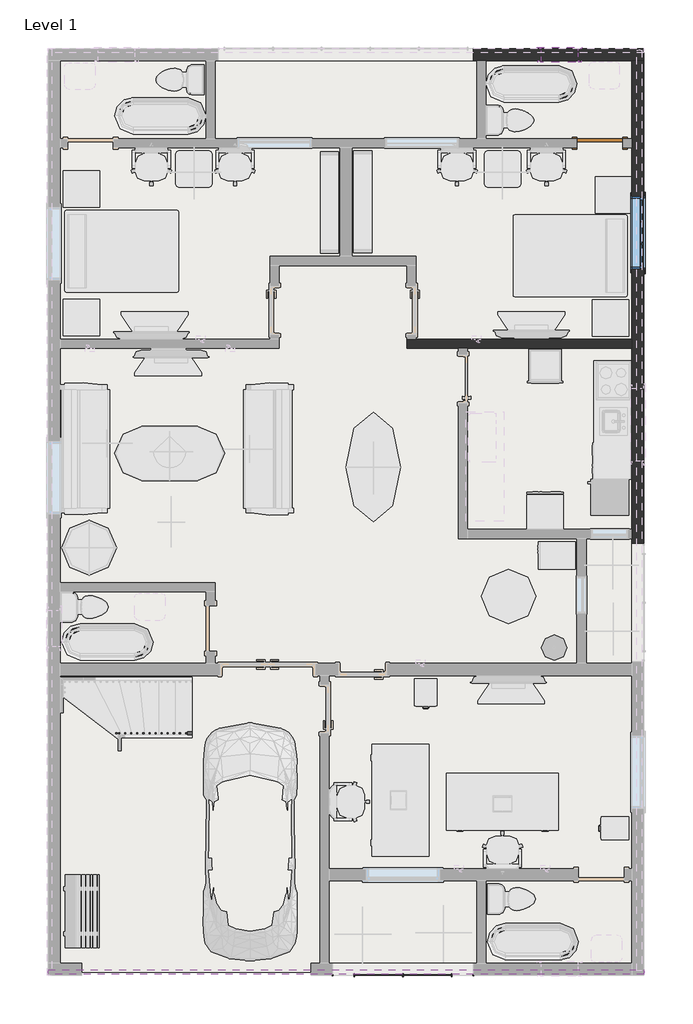
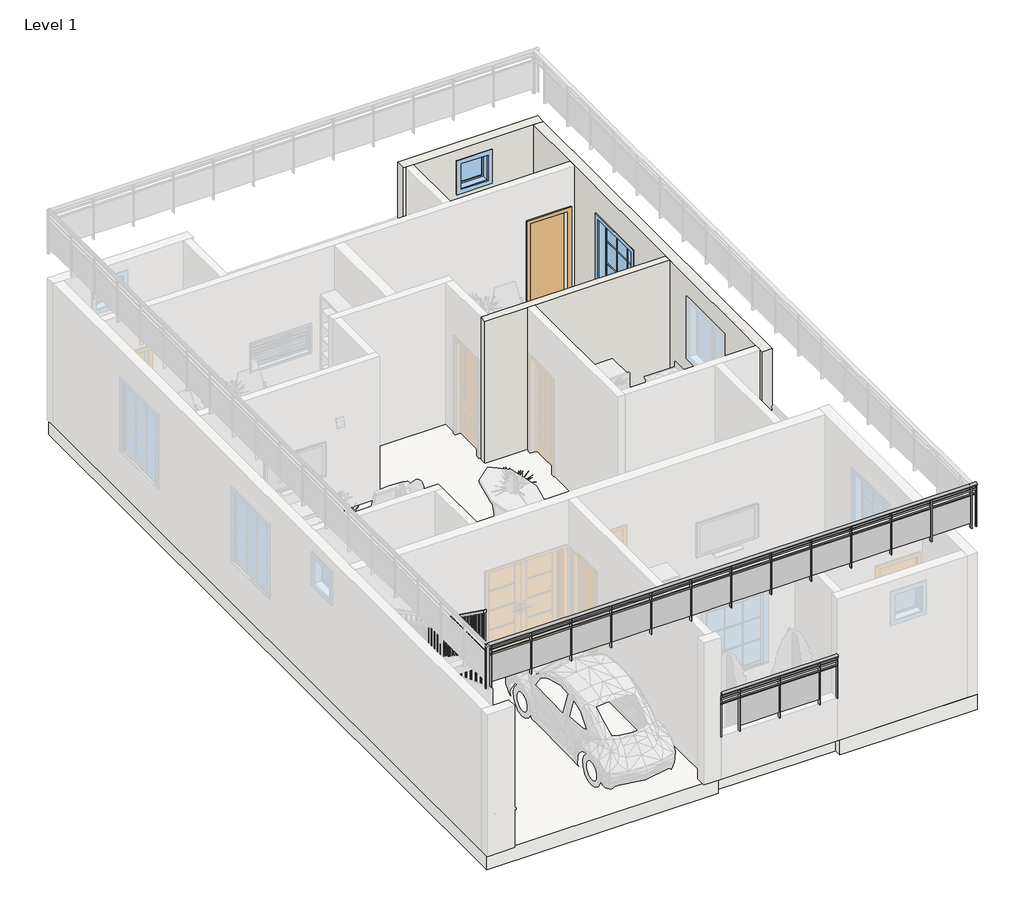
# One storey, part 2 of 5: 3 railings, 3 walls, 2 windows, 1 door, 1 slab.
"""IFC4 building model written with IfcOpenShell, lengths in millimetres."""

from ifc_helpers import new_model, si_unit, point, frame, origin, place, context, project, spatial, polyline, ellipse_curve, trimmed, outline, extrude, faceted_brep, transform, mapped, element, save
from ifc_brep_helpers import plane_surface, extruded_surface, advanced_brep
from components import door_a9addea7, window_cfa1ffdd, window_e41d21a6

model = new_model("IFC4")

# Units and contexts
model_context = context("Model", 3, world=origin())
ifc_project = project(units=[si_unit("LENGTHUNIT", "METRE", prefix="MILLI")], contexts=[model_context])

# Site, building, storey
site = spatial("IfcSite", under=ifc_project)
building = spatial("IfcBuilding", under=site)
storey = spatial("IfcBuildingStorey", under=building, Name="Level 1", Elevation=0.0)

# Door
placement = place(None, origin())
door_shape = door_a9addea7(model_context)
element("IfcDoor", 1, ObjectType="Single-Flush : 30\" x 84\"", at=placement, inside=storey, context=model_context, shape_type="MappedRepresentation", body=[
    mapped(door_shape, transform((1921.0042848, 14492.9691167, 0.0), x_axis=(1.0, 0.0, 0.0), y_axis=(0.0, 1.0, 0.0), z_axis=(0.0, 0.0, 1.0))),
])

# Railings
element("IfcRailing", 2, ObjectType="Glass Panel - Bottom Fill", at=placement, inside=storey, context=model_context, shape_type="SolidModel", body=[
    advanced_brep(
    [(-2549.3957152, 637.2691167, 1828.8), (-2549.3957152, 561.0691167, 1828.8), (-187.1957152, 637.2691167, 1828.8), (-187.1957152, 561.0691167, 1828.8)],
    [
        (0, 1, ellipse_curve(frame((-2549.3957152, 599.1691167, 1828.8), z_axis=(-1.0, 0.0, 0.0), x_axis=(0.0, -1.0, 0.0)), 38.1, 28.575)),
        (1, 0, ellipse_curve(frame((-2549.3957152, 599.1691167, 1828.8), z_axis=(-1.0, 0.0, 0.0), x_axis=(0.0, -1.0, 0.0)), 38.1, 28.575)),
        (2, 3, ellipse_curve(frame((-187.1957152, 599.1691167, 1828.8), z_axis=(1.0, 0.0, 0.0), x_axis=(0.0, -1.0, 0.0)), 38.1, 28.575)),
        (3, 2, ellipse_curve(frame((-187.1957152, 599.1691167, 1828.8), z_axis=(1.0, 0.0, 0.0), x_axis=(0.0, -1.0, 0.0)), 38.1, 28.575)),
        (0, 2),
        (3, 1),
    ],
    [
        plane_surface(frame((-2549.3957152, 599.1691167, 1828.8), z_axis=(-1.0, 0.0, 0.0), x_axis=(0.0, 1.0, 0.0))),
        plane_surface(frame((-187.1957152, 599.1691167, 1828.8), z_axis=(1.0, 0.0, 0.0), x_axis=(0.0, 1.0, 0.0))),
        extruded_surface(trimmed(ellipse_curve(frame((-187.1957152, 599.1691167, 1828.8), z_axis=(-1.0, 0.0, 0.0), x_axis=(0.0, -1.0, 0.0)), 38.1, 28.575), [point((-187.1957152, 637.2691167, 1828.8))], [point((-187.1957152, 561.0691167, 1828.8))], True, "CARTESIAN"), (-2362.2, 0.0, 0.0), 2362.2),
        extruded_surface(trimmed(ellipse_curve(frame((-187.1957152, 599.1691167, 1828.8), z_axis=(-1.0, 0.0, 0.0), x_axis=(0.0, -1.0, 0.0)), 38.1, 28.575), [point((-187.1957152, 561.0691167, 1828.8))], [point((-187.1957152, 637.2691167, 1828.8))], True, "CARTESIAN"), (-2362.2, 0.0, 0.0), 2362.2),
    ],
    [
        (0, [[1, 2]]),
        (1, [[3, 4]]),
        (2, [[-1, 5, -4, 6]]),
        (3, [[-2, -6, -3, -5]]),
    ],
),
    extrude(outline(polyline([(-2549.3957152, 586.4691167), (-2549.3957152, 611.8691167), (-187.1957152, 611.8691167), (-187.1957152, 586.4691167), (-2549.3957152, 586.4691167)])), frame((0.0, 0.0, 1714.5), z_axis=(0.0, 0.0, 1.0), x_axis=(1.0, 0.0, 0.0)), (0.0, 0.0, 1.0), 25.4),
    extrude(outline(polyline([(-2549.3957152, 586.4691167), (-2549.3957152, 611.8691167), (-187.1957152, 611.8691167), (-187.1957152, 586.4691167), (-2549.3957152, 586.4691167)])), frame((0.0, 0.0, 1612.9), z_axis=(0.0, 0.0, 1.0), x_axis=(1.0, 0.0, 0.0)), (0.0, 0.0, 1.0), 25.4),
    extrude(outline(polyline([(-561.8457152, 573.7691167), (-561.8457152, 624.5691167), (-549.1457152, 624.5691167), (-549.1457152, 573.7691167), (-561.8457152, 573.7691167)])), frame((0.0, 0.0, 914.4), z_axis=(0.0, 0.0, 1.0), x_axis=(1.0, 0.0, 0.0)), (0.0, 0.0, 1.0), 885.6788223),
    extrude(outline(polyline([(-1368.2957152, 605.7042737), (-555.4957152, 605.7042737), (-555.4957152, 599.3542737), (-1368.2957152, 599.3542737), (-1368.2957152, 605.7042737)])), frame((0.0, 0.0, 1016.0), z_axis=(0.0, 0.0, 1.0), x_axis=(1.0, 0.0, 0.0)), (0.0, 0.0, 1.0), 596.9),
    extrude(outline(polyline([(-1374.6457152, 573.7691167), (-1374.6457152, 624.5691167), (-1361.9457152, 624.5691167), (-1361.9457152, 573.7691167), (-1374.6457152, 573.7691167)])), frame((0.0, 0.0, 914.4), z_axis=(0.0, 0.0, 1.0), x_axis=(1.0, 0.0, 0.0)), (0.0, 0.0, 1.0), 885.6788223),
    extrude(outline(polyline([(-2181.0957152, 605.7042737), (-1368.2957152, 605.7042737), (-1368.2957152, 599.3542737), (-2181.0957152, 599.3542737), (-2181.0957152, 605.7042737)])), frame((0.0, 0.0, 1016.0), z_axis=(0.0, 0.0, 1.0), x_axis=(1.0, 0.0, 0.0)), (0.0, 0.0, 1.0), 596.9),
    extrude(outline(polyline([(-2187.4457152, 573.7691167), (-2187.4457152, 624.5691167), (-2174.7457152, 624.5691167), (-2174.7457152, 573.7691167), (-2187.4457152, 573.7691167)])), frame((0.0, 0.0, 914.4), z_axis=(0.0, 0.0, 1.0), x_axis=(1.0, 0.0, 0.0)), (0.0, 0.0, 1.0), 885.6788223),
    extrude(outline(polyline([(-199.8957152, 589.6441167), (-199.8957152, 608.6941167), (-180.8457152, 608.6941167), (-180.8457152, 589.6441167), (-199.8957152, 589.6441167)])), frame((0.0, 0.0, 914.4), z_axis=(0.0, 0.0, 1.0), x_axis=(1.0, 0.0, 0.0)), (0.0, 0.0, 1.0), 885.6788223),
    extrude(outline(polyline([(-2555.7457152, 589.6441167), (-2555.7457152, 608.6941167), (-2536.6957152, 608.6941167), (-2536.6957152, 589.6441167), (-2555.7457152, 589.6441167)])), frame((0.0, 0.0, 914.4), z_axis=(0.0, 0.0, 1.0), x_axis=(1.0, 0.0, 0.0)), (0.0, 0.0, 1.0), 885.6788223),
])
element("IfcRailing", 3, ObjectType="Glass Panel - Bottom Fill", at=placement, inside=storey, context=model_context, shape_type="SolidModel", body=[
    advanced_brep(
    [(-7299.1957152, 688.0691167, 4495.8), (-7299.1957152, 611.8691167, 4495.8), (2657.6042848, 688.0691167, 4495.8), (2657.6042848, 611.8691167, 4495.8)],
    [
        (0, 1, ellipse_curve(frame((-7299.1957152, 649.9691167, 4495.8), z_axis=(-1.0, 0.0, 0.0), x_axis=(0.0, -1.0, 0.0)), 38.1, 28.575)),
        (1, 0, ellipse_curve(frame((-7299.1957152, 649.9691167, 4495.8), z_axis=(-1.0, 0.0, 0.0), x_axis=(0.0, -1.0, 0.0)), 38.1, 28.575)),
        (2, 3, ellipse_curve(frame((2657.6042848, 649.9691167, 4495.8), z_axis=(1.0, 0.0, 0.0), x_axis=(0.0, -1.0, 0.0)), 38.1, 28.575)),
        (3, 2, ellipse_curve(frame((2657.6042848, 649.9691167, 4495.8), z_axis=(1.0, 0.0, 0.0), x_axis=(0.0, -1.0, 0.0)), 38.1, 28.575)),
        (0, 2),
        (3, 1),
    ],
    [
        plane_surface(frame((-7299.1957152, 649.9691167, 4495.8), z_axis=(-1.0, 0.0, 0.0), x_axis=(0.0, 1.0, 0.0))),
        plane_surface(frame((2657.6042848, 649.9691167, 4495.8), z_axis=(1.0, 0.0, 0.0), x_axis=(0.0, 1.0, 0.0))),
        extruded_surface(trimmed(ellipse_curve(frame((2657.6042848, 649.9691167, 4495.8), z_axis=(-1.0, 0.0, 0.0), x_axis=(0.0, -1.0, 0.0)), 38.1, 28.575), [point((2657.6042848, 688.0691167, 4495.8))], [point((2657.6042848, 611.8691167, 4495.8))], True, "CARTESIAN"), (-9956.800000000001, 0.0, 0.0), 9956.800000000001),
        extruded_surface(trimmed(ellipse_curve(frame((2657.6042848, 649.9691167, 4495.8), z_axis=(-1.0, 0.0, 0.0), x_axis=(0.0, -1.0, 0.0)), 38.1, 28.575), [point((2657.6042848, 611.8691167, 4495.8))], [point((2657.6042848, 688.0691167, 4495.8))], True, "CARTESIAN"), (-9956.800000000001, 0.0, 0.0), 9956.800000000001),
    ],
    [
        (0, [[1, 2]]),
        (1, [[3, 4]]),
        (2, [[-1, 5, -4, 6]]),
        (3, [[-2, -6, -3, -5]]),
    ],
),
    extrude(outline(polyline([(-7299.1957152, 637.2691167), (-7299.1957152, 662.6691167), (2657.6042848, 662.6691167), (2657.6042848, 637.2691167), (-7299.1957152, 637.2691167)])), frame((0.0, 0.0, 4381.5), z_axis=(0.0, 0.0, 1.0), x_axis=(1.0, 0.0, 0.0)), (0.0, 0.0, 1.0), 25.4),
    extrude(outline(polyline([(-7299.1957152, 637.2691167), (-7299.1957152, 662.6691167), (2657.6042848, 662.6691167), (2657.6042848, 637.2691167), (-7299.1957152, 637.2691167)])), frame((0.0, 0.0, 4279.9), z_axis=(0.0, 0.0, 1.0), x_axis=(1.0, 0.0, 0.0)), (0.0, 0.0, 1.0), 25.4),
    extrude(outline(polyline([(2549.6542848, 624.5691167), (2549.6542848, 675.3691167), (2562.3542848, 675.3691167), (2562.3542848, 624.5691167), (2549.6542848, 624.5691167)])), frame((0.0, 0.0, 3581.4), z_axis=(0.0, 0.0, 1.0), x_axis=(1.0, 0.0, 0.0)), (0.0, 0.0, 1.0), 885.6788223),
    extrude(outline(polyline([(1743.2042848, 656.5042737), (2556.0042848, 656.5042737), (2556.0042848, 650.1542737), (1743.2042848, 650.1542737), (1743.2042848, 656.5042737)])), frame((0.0, 0.0, 3683.0), z_axis=(0.0, 0.0, 1.0), x_axis=(1.0, 0.0, 0.0)), (0.0, 0.0, 1.0), 596.9),
    extrude(outline(polyline([(1736.8542848, 624.5691167), (1736.8542848, 675.3691167), (1749.5542848, 675.3691167), (1749.5542848, 624.5691167), (1736.8542848, 624.5691167)])), frame((0.0, 0.0, 3581.4), z_axis=(0.0, 0.0, 1.0), x_axis=(1.0, 0.0, 0.0)), (0.0, 0.0, 1.0), 885.6788223),
    extrude(outline(polyline([(930.4042848, 656.5042737), (1743.2042848, 656.5042737), (1743.2042848, 650.1542737), (930.4042848, 650.1542737), (930.4042848, 656.5042737)])), frame((0.0, 0.0, 3683.0), z_axis=(0.0, 0.0, 1.0), x_axis=(1.0, 0.0, 0.0)), (0.0, 0.0, 1.0), 596.9),
    extrude(outline(polyline([(924.0542848, 624.5691167), (924.0542848, 675.3691167), (936.7542848, 675.3691167), (936.7542848, 624.5691167), (924.0542848, 624.5691167)])), frame((0.0, 0.0, 3581.4), z_axis=(0.0, 0.0, 1.0), x_axis=(1.0, 0.0, 0.0)), (0.0, 0.0, 1.0), 885.6788223),
    extrude(outline(polyline([(117.6042848, 656.5042737), (930.4042848, 656.5042737), (930.4042848, 650.1542737), (117.6042848, 650.1542737), (117.6042848, 656.5042737)])), frame((0.0, 0.0, 3683.0), z_axis=(0.0, 0.0, 1.0), x_axis=(1.0, 0.0, 0.0)), (0.0, 0.0, 1.0), 596.9),
    extrude(outline(polyline([(111.2542848, 624.5691167), (111.2542848, 675.3691167), (123.9542848, 675.3691167), (123.9542848, 624.5691167), (111.2542848, 624.5691167)])), frame((0.0, 0.0, 3581.4), z_axis=(0.0, 0.0, 1.0), x_axis=(1.0, 0.0, 0.0)), (0.0, 0.0, 1.0), 885.6788223),
    extrude(outline(polyline([(-695.1957152, 656.5042737), (117.6042848, 656.5042737), (117.6042848, 650.1542737), (-695.1957152, 650.1542737), (-695.1957152, 656.5042737)])), frame((0.0, 0.0, 3683.0), z_axis=(0.0, 0.0, 1.0), x_axis=(1.0, 0.0, 0.0)), (0.0, 0.0, 1.0), 596.9),
    extrude(outline(polyline([(-701.5457152, 624.5691167), (-701.5457152, 675.3691167), (-688.8457152, 675.3691167), (-688.8457152, 624.5691167), (-701.5457152, 624.5691167)])), frame((0.0, 0.0, 3581.4), z_axis=(0.0, 0.0, 1.0), x_axis=(1.0, 0.0, 0.0)), (0.0, 0.0, 1.0), 885.6788223),
    extrude(outline(polyline([(-1507.9957152, 656.5042737), (-695.1957152, 656.5042737), (-695.1957152, 650.1542737), (-1507.9957152, 650.1542737), (-1507.9957152, 656.5042737)])), frame((0.0, 0.0, 3683.0), z_axis=(0.0, 0.0, 1.0), x_axis=(1.0, 0.0, 0.0)), (0.0, 0.0, 1.0), 596.9),
    extrude(outline(polyline([(-1514.3457152, 624.5691167), (-1514.3457152, 675.3691167), (-1501.6457152, 675.3691167), (-1501.6457152, 624.5691167), (-1514.3457152, 624.5691167)])), frame((0.0, 0.0, 3581.4), z_axis=(0.0, 0.0, 1.0), x_axis=(1.0, 0.0, 0.0)), (0.0, 0.0, 1.0), 885.6788223),
    extrude(outline(polyline([(-2320.7957152, 656.5042737), (-1507.9957152, 656.5042737), (-1507.9957152, 650.1542737), (-2320.7957152, 650.1542737), (-2320.7957152, 656.5042737)])), frame((0.0, 0.0, 3683.0), z_axis=(0.0, 0.0, 1.0), x_axis=(1.0, 0.0, 0.0)), (0.0, 0.0, 1.0), 596.9),
    extrude(outline(polyline([(-2327.1457152, 624.5691167), (-2327.1457152, 675.3691167), (-2314.4457152, 675.3691167), (-2314.4457152, 624.5691167), (-2327.1457152, 624.5691167)])), frame((0.0, 0.0, 3581.4), z_axis=(0.0, 0.0, 1.0), x_axis=(1.0, 0.0, 0.0)), (0.0, 0.0, 1.0), 885.6788223),
    extrude(outline(polyline([(-3133.5957152, 656.5042737), (-2320.7957152, 656.5042737), (-2320.7957152, 650.1542737), (-3133.5957152, 650.1542737), (-3133.5957152, 656.5042737)])), frame((0.0, 0.0, 3683.0), z_axis=(0.0, 0.0, 1.0), x_axis=(1.0, 0.0, 0.0)), (0.0, 0.0, 1.0), 596.9),
    extrude(outline(polyline([(-3139.9457152, 624.5691167), (-3139.9457152, 675.3691167), (-3127.2457152, 675.3691167), (-3127.2457152, 624.5691167), (-3139.9457152, 624.5691167)])), frame((0.0, 0.0, 3581.4), z_axis=(0.0, 0.0, 1.0), x_axis=(1.0, 0.0, 0.0)), (0.0, 0.0, 1.0), 885.6788223),
    extrude(outline(polyline([(-3946.3957152, 656.5042737), (-3133.5957152, 656.5042737), (-3133.5957152, 650.1542737), (-3946.3957152, 650.1542737), (-3946.3957152, 656.5042737)])), frame((0.0, 0.0, 3683.0), z_axis=(0.0, 0.0, 1.0), x_axis=(1.0, 0.0, 0.0)), (0.0, 0.0, 1.0), 596.9),
    extrude(outline(polyline([(-3952.7457152, 624.5691167), (-3952.7457152, 675.3691167), (-3940.0457152, 675.3691167), (-3940.0457152, 624.5691167), (-3952.7457152, 624.5691167)])), frame((0.0, 0.0, 3581.4), z_axis=(0.0, 0.0, 1.0), x_axis=(1.0, 0.0, 0.0)), (0.0, 0.0, 1.0), 885.6788223),
    extrude(outline(polyline([(-4759.1957152, 656.5042737), (-3946.3957152, 656.5042737), (-3946.3957152, 650.1542737), (-4759.1957152, 650.1542737), (-4759.1957152, 656.5042737)])), frame((0.0, 0.0, 3683.0), z_axis=(0.0, 0.0, 1.0), x_axis=(1.0, 0.0, 0.0)), (0.0, 0.0, 1.0), 596.9),
    extrude(outline(polyline([(-4765.5457152, 624.5691167), (-4765.5457152, 675.3691167), (-4752.8457152, 675.3691167), (-4752.8457152, 624.5691167), (-4765.5457152, 624.5691167)])), frame((0.0, 0.0, 3581.4), z_axis=(0.0, 0.0, 1.0), x_axis=(1.0, 0.0, 0.0)), (0.0, 0.0, 1.0), 885.6788223),
    extrude(outline(polyline([(-5571.9957152, 656.5042737), (-4759.1957152, 656.5042737), (-4759.1957152, 650.1542737), (-5571.9957152, 650.1542737), (-5571.9957152, 656.5042737)])), frame((0.0, 0.0, 3683.0), z_axis=(0.0, 0.0, 1.0), x_axis=(1.0, 0.0, 0.0)), (0.0, 0.0, 1.0), 596.9),
    extrude(outline(polyline([(-5578.3457152, 624.5691167), (-5578.3457152, 675.3691167), (-5565.6457152, 675.3691167), (-5565.6457152, 624.5691167), (-5578.3457152, 624.5691167)])), frame((0.0, 0.0, 3581.4), z_axis=(0.0, 0.0, 1.0), x_axis=(1.0, 0.0, 0.0)), (0.0, 0.0, 1.0), 885.6788223),
    extrude(outline(polyline([(-6384.7957152, 656.5042737), (-5571.9957152, 656.5042737), (-5571.9957152, 650.1542737), (-6384.7957152, 650.1542737), (-6384.7957152, 656.5042737)])), frame((0.0, 0.0, 3683.0), z_axis=(0.0, 0.0, 1.0), x_axis=(1.0, 0.0, 0.0)), (0.0, 0.0, 1.0), 596.9),
    extrude(outline(polyline([(-6391.1457152, 624.5691167), (-6391.1457152, 675.3691167), (-6378.4457152, 675.3691167), (-6378.4457152, 624.5691167), (-6391.1457152, 624.5691167)])), frame((0.0, 0.0, 3581.4), z_axis=(0.0, 0.0, 1.0), x_axis=(1.0, 0.0, 0.0)), (0.0, 0.0, 1.0), 885.6788223),
    extrude(outline(polyline([(-7197.5957152, 656.5042737), (-6384.7957152, 656.5042737), (-6384.7957152, 650.1542737), (-7197.5957152, 650.1542737), (-7197.5957152, 656.5042737)])), frame((0.0, 0.0, 3683.0), z_axis=(0.0, 0.0, 1.0), x_axis=(1.0, 0.0, 0.0)), (0.0, 0.0, 1.0), 596.9),
    extrude(outline(polyline([(-7203.9457152, 624.5691167), (-7203.9457152, 675.3691167), (-7191.2457152, 675.3691167), (-7191.2457152, 624.5691167), (-7203.9457152, 624.5691167)])), frame((0.0, 0.0, 3581.4), z_axis=(0.0, 0.0, 1.0), x_axis=(1.0, 0.0, 0.0)), (0.0, 0.0, 1.0), 885.6788223),
    extrude(outline(polyline([(2644.9042848, 640.4441167), (2644.9042848, 659.4941167), (2663.9542848, 659.4941167), (2663.9542848, 640.4441167), (2644.9042848, 640.4441167)])), frame((0.0, 0.0, 3581.4), z_axis=(0.0, 0.0, 1.0), x_axis=(1.0, 0.0, 0.0)), (0.0, 0.0, 1.0), 885.6788223),
    extrude(outline(polyline([(-7305.5457152, 640.4441167), (-7305.5457152, 659.4941167), (-7286.4957152, 659.4941167), (-7286.4957152, 640.4441167), (-7305.5457152, 640.4441167)])), frame((0.0, 0.0, 3581.4), z_axis=(0.0, 0.0, 1.0), x_axis=(1.0, 0.0, 0.0)), (0.0, 0.0, 1.0), 885.6788223),
])
element("IfcRailing", 4, ObjectType="Handrail - Rectangular", at=placement, inside=storey, context=model_context, shape_type="SolidModel", body=[
    faceted_brep([(-4892.6027934, 4612.3691167, 1210.6955174), (-4892.6027934, 4612.3691167, 1146.9597126), (-4892.6027934, 4663.1691167, 1146.9597126), (-4892.6027934, 4663.1691167, 1210.6955174), (-6054.5957152, 4612.3691167, 2091.1504574), (-6105.3957152, 4612.3691167, 2065.9063766), (-6105.3957152, 4663.1691167, 2065.9063766), (-6054.5957152, 4663.1691167, 2091.1504574), (-6054.5957152, 4612.3691167, 2301.2616873), (-6105.3957152, 4612.3691167, 2250.4616873), (-6105.3957152, 4663.1691167, 2250.4616873), (-6054.5957152, 4663.1691167, 2301.2616873), (-6130.7957152, 4612.3691167, 2301.2616873), (-6130.7957152, 4612.3691167, 2250.4616873), (-6181.5957152, 4663.1691167, 2250.4616873), (-6181.5957152, 4663.1691167, 2301.2616873), (-6130.7957152, 4536.1691167, 2301.2616873), (-6130.7957152, 4519.8580772, 2250.4616873), (-6181.5957152, 4519.8580772, 2250.4616873), (-6181.5957152, 4536.1691167, 2301.2616873), (-6130.7957152, 2646.197182, 3654.4449888), (-6181.5957152, 2646.197182, 3654.4449888), (-6181.5957152, 2646.197182, 3591.9666004), (-6130.7957152, 2646.197182, 3591.9666004)], [[[0, 1, 2, 3]], [[1, 0, 4, 5]], [[2, 1, 5, 6]], [[3, 2, 6, 7]], [[0, 3, 7, 4]], [[5, 4, 8, 9]], [[6, 5, 9, 10]], [[7, 6, 10, 11]], [[4, 7, 11, 8]], [[9, 8, 12, 13]], [[10, 9, 13, 14]], [[11, 10, 14, 15]], [[8, 11, 15, 12]], [[13, 12, 16, 17]], [[14, 13, 17, 18]], [[15, 14, 18, 19]], [[12, 15, 19, 16]], [[20, 21, 22, 23]], [[17, 16, 20, 23]], [[18, 17, 23, 22]], [[19, 18, 22, 21]], [[16, 19, 21, 20]]]),
    extrude(outline(polyline([(2716.8941167, 3541.3489644), (2716.8941167, 2540.0), (2697.8441167, 2540.0), (2697.8441167, 3554.9883955), (2716.8941167, 3541.3489644)])), frame((-6165.7207152, 0.0, 0.0), z_axis=(1.0, 0.0, 0.0), x_axis=(0.0, 1.0, 0.0)), (0.0, 0.0, 1.0), 19.05),
    extrude(outline(polyline([(2818.4941167, 3468.6053322), (2818.4941167, 2540.0), (2799.4441167, 2540.0), (2799.4441167, 3482.2447632), (2818.4941167, 3468.6053322)])), frame((-6165.7207152, 0.0, 0.0), z_axis=(1.0, 0.0, 0.0), x_axis=(0.0, 1.0, 0.0)), (0.0, 0.0, 1.0), 19.05),
    extrude(outline(polyline([(2920.0941167, 3395.8616999), (2920.0941167, 2540.0), (2901.0441167, 2540.0), (2901.0441167, 3409.5011309), (2920.0941167, 3395.8616999)])), frame((-6165.7207152, 0.0, 0.0), z_axis=(1.0, 0.0, 0.0), x_axis=(0.0, 1.0, 0.0)), (0.0, 0.0, 1.0), 19.05),
    extrude(outline(polyline([(3021.6941167, 3323.1180676), (3021.6941167, 2370.6666667), (3002.6441167, 2370.6666667), (3002.6441167, 3336.7574987), (3021.6941167, 3323.1180676)])), frame((-6165.7207152, 0.0, 0.0), z_axis=(1.0, 0.0, 0.0), x_axis=(0.0, 1.0, 0.0)), (0.0, 0.0, 1.0), 19.05),
    extrude(outline(polyline([(3123.2941167, 3250.3744353), (3123.2941167, 2370.6666667), (3104.2441167, 2370.6666667), (3104.2441167, 3264.0138664), (3123.2941167, 3250.3744353)])), frame((-6165.7207152, 0.0, 0.0), z_axis=(1.0, 0.0, 0.0), x_axis=(0.0, 1.0, 0.0)), (0.0, 0.0, 1.0), 19.05),
    extrude(outline(polyline([(3224.8941167, 3177.6308031), (3224.8941167, 2201.3333333), (3205.8441167, 2201.3333333), (3205.8441167, 3191.2702341), (3224.8941167, 3177.6308031)])), frame((-6165.7207152, 0.0, 0.0), z_axis=(1.0, 0.0, 0.0), x_axis=(0.0, 1.0, 0.0)), (0.0, 0.0, 1.0), 19.05),
    extrude(outline(polyline([(3326.4941167, 3104.8871708), (3326.4941167, 2201.3333333), (3307.4441167, 2201.3333333), (3307.4441167, 3118.5266018), (3326.4941167, 3104.8871708)])), frame((-6165.7207152, 0.0, 0.0), z_axis=(1.0, 0.0, 0.0), x_axis=(0.0, 1.0, 0.0)), (0.0, 0.0, 1.0), 19.05),
    extrude(outline(polyline([(3428.0941167, 3032.1435385), (3428.0941167, 2201.3333333), (3409.0441167, 2201.3333333), (3409.0441167, 3045.7829696), (3428.0941167, 3032.1435385)])), frame((-6165.7207152, 0.0, 0.0), z_axis=(1.0, 0.0, 0.0), x_axis=(0.0, 1.0, 0.0)), (0.0, 0.0, 1.0), 19.05),
    extrude(outline(polyline([(3529.6941167, 2959.3999062), (3529.6941167, 2032.0), (3510.6441167, 2032.0), (3510.6441167, 2973.0393373), (3529.6941167, 2959.3999062)])), frame((-6165.7207152, 0.0, 0.0), z_axis=(1.0, 0.0, 0.0), x_axis=(0.0, 1.0, 0.0)), (0.0, 0.0, 1.0), 19.05),
    extrude(outline(polyline([(3631.2941167, 2886.656274), (3631.2941167, 2032.0), (3612.2441167, 2032.0), (3612.2441167, 2900.295705), (3631.2941167, 2886.656274)])), frame((-6165.7207152, 0.0, 0.0), z_axis=(1.0, 0.0, 0.0), x_axis=(0.0, 1.0, 0.0)), (0.0, 0.0, 1.0), 19.05),
    extrude(outline(polyline([(3732.8941167, 2813.9126417), (3732.8941167, 2032.0), (3713.8441167, 2032.0), (3713.8441167, 2827.5520727), (3732.8941167, 2813.9126417)])), frame((-6165.7207152, 0.0, 0.0), z_axis=(1.0, 0.0, 0.0), x_axis=(0.0, 1.0, 0.0)), (0.0, 0.0, 1.0), 19.05),
    extrude(outline(polyline([(3834.4941167, 2741.1690094), (3834.4941167, 1862.6666667), (3815.4441167, 1862.6666667), (3815.4441167, 2754.8084405), (3834.4941167, 2741.1690094)])), frame((-6165.7207152, 0.0, 0.0), z_axis=(1.0, 0.0, 0.0), x_axis=(0.0, 1.0, 0.0)), (0.0, 0.0, 1.0), 19.05),
    extrude(outline(polyline([(3936.0941167, 2668.4253771), (3936.0941167, 1862.6666667), (3917.0441167, 1862.6666667), (3917.0441167, 2682.0648082), (3936.0941167, 2668.4253771)])), frame((-6165.7207152, 0.0, 0.0), z_axis=(1.0, 0.0, 0.0), x_axis=(0.0, 1.0, 0.0)), (0.0, 0.0, 1.0), 19.05),
    extrude(outline(polyline([(4037.6941167, 2595.6817449), (4037.6941167, 1693.3333333), (4018.6441167, 1693.3333333), (4018.6441167, 2609.3211759), (4037.6941167, 2595.6817449)])), frame((-6165.7207152, 0.0, 0.0), z_axis=(1.0, 0.0, 0.0), x_axis=(0.0, 1.0, 0.0)), (0.0, 0.0, 1.0), 19.05),
    extrude(outline(polyline([(4139.2941167, 2522.9381126), (4139.2941167, 1693.3333333), (4120.2441167, 1693.3333333), (4120.2441167, 2536.5775436), (4139.2941167, 2522.9381126)])), frame((-6165.7207152, 0.0, 0.0), z_axis=(1.0, 0.0, 0.0), x_axis=(0.0, 1.0, 0.0)), (0.0, 0.0, 1.0), 19.05),
    extrude(outline(polyline([(4240.8941167, 2450.1944803), (4240.8941167, 1524.0), (4221.8441167, 1524.0), (4221.8441167, 2463.8339114), (4240.8941167, 2450.1944803)])), frame((-6165.7207152, 0.0, 0.0), z_axis=(1.0, 0.0, 0.0), x_axis=(0.0, 1.0, 0.0)), (0.0, 0.0, 1.0), 19.05),
    extrude(outline(polyline([(4342.4941167, 2377.450848), (4342.4941167, 1524.0), (4323.4441167, 1524.0), (4323.4441167, 2391.0902791), (4342.4941167, 2377.450848)])), frame((-6165.7207152, 0.0, 0.0), z_axis=(1.0, 0.0, 0.0), x_axis=(0.0, 1.0, 0.0)), (0.0, 0.0, 1.0), 19.05),
    extrude(outline(polyline([(4444.0941167, 2304.7072158), (4444.0941167, 1354.6666667), (4425.0441167, 1354.6666667), (4425.0441167, 2318.3466468), (4444.0941167, 2304.7072158)])), frame((-6165.7207152, 0.0, 0.0), z_axis=(1.0, 0.0, 0.0), x_axis=(0.0, 1.0, 0.0)), (0.0, 0.0, 1.0), 19.05),
    extrude(outline(polyline([(-6146.6707152, 4545.6941167), (-6146.6707152, 4526.6441167), (-6165.7207152, 4526.6441167), (-6165.7207152, 4545.6941167), (-6146.6707152, 4545.6941167)])), frame((0.0, 0.0, 1354.6666667), z_axis=(0.0, 0.0, 1.0), x_axis=(1.0, 0.0, 0.0)), (0.0, 0.0, 1.0), 895.7950207),
    extrude(outline(polyline([(2077.8270257, -6121.3277934), (1185.3333333, -6121.3277934), (1185.3333333, -6102.2777934), (2063.3926292, -6102.2777934), (2077.8270257, -6121.3277934)])), frame((0.0, 4628.2441167, 0.0), z_axis=(0.0, 1.0, 0.0), x_axis=(0.0, 0.0, 1.0)), (0.0, 0.0, 1.0), 19.05),
    extrude(outline(polyline([(2000.994841, -6019.7277934), (1016.0, -6019.7277934), (1016.0, -6000.6777934), (1986.5604445, -6000.6777934), (2000.994841, -6019.7277934)])), frame((0.0, 4628.2441167, 0.0), z_axis=(0.0, 1.0, 0.0), x_axis=(0.0, 0.0, 1.0)), (0.0, 0.0, 1.0), 19.05),
    extrude(outline(polyline([(1924.0113928, -5918.1277934), (1016.0, -5918.1277934), (1016.0, -5899.0777934), (1909.5769963, -5899.0777934), (1924.0113928, -5918.1277934)])), frame((0.0, 4628.2441167, 0.0), z_axis=(0.0, 1.0, 0.0), x_axis=(0.0, 0.0, 1.0)), (0.0, 0.0, 1.0), 19.05),
    extrude(outline(polyline([(1847.0279446, -5816.5277934), (846.6666667, -5816.5277934), (846.6666667, -5797.4777934), (1832.5935481, -5797.4777934), (1847.0279446, -5816.5277934)])), frame((0.0, 4628.2441167, 0.0), z_axis=(0.0, 1.0, 0.0), x_axis=(0.0, 0.0, 1.0)), (0.0, 0.0, 1.0), 19.05),
    extrude(outline(polyline([(1770.0444964, -5714.9277934), (846.6666667, -5714.9277934), (846.6666667, -5695.8777934), (1755.6100999, -5695.8777934), (1770.0444964, -5714.9277934)])), frame((0.0, 4628.2441167, 0.0), z_axis=(0.0, 1.0, 0.0), x_axis=(0.0, 0.0, 1.0)), (0.0, 0.0, 1.0), 19.05),
    extrude(outline(polyline([(1693.0610482, -5613.3277934), (677.3333333, -5613.3277934), (677.3333333, -5594.2777934), (1678.6266517, -5594.2777934), (1693.0610482, -5613.3277934)])), frame((0.0, 4628.2441167, 0.0), z_axis=(0.0, 1.0, 0.0), x_axis=(0.0, 0.0, 1.0)), (0.0, 0.0, 1.0), 19.05),
    extrude(outline(polyline([(1616.0776, -5511.7277934), (677.3333333, -5511.7277934), (677.3333333, -5492.6777934), (1601.6432035, -5492.6777934), (1616.0776, -5511.7277934)])), frame((0.0, 4628.2441167, 0.0), z_axis=(0.0, 1.0, 0.0), x_axis=(0.0, 0.0, 1.0)), (0.0, 0.0, 1.0), 19.05),
    extrude(outline(polyline([(1539.0941518, -5410.1277934), (508.0, -5410.1277934), (508.0, -5391.0777934), (1524.6597553, -5391.0777934), (1539.0941518, -5410.1277934)])), frame((0.0, 4628.2441167, 0.0), z_axis=(0.0, 1.0, 0.0), x_axis=(0.0, 0.0, 1.0)), (0.0, 0.0, 1.0), 19.05),
    extrude(outline(polyline([(1462.1107036, -5308.5277934), (508.0, -5308.5277934), (508.0, -5289.4777934), (1447.6763071, -5289.4777934), (1462.1107036, -5308.5277934)])), frame((0.0, 4628.2441167, 0.0), z_axis=(0.0, 1.0, 0.0), x_axis=(0.0, 0.0, 1.0)), (0.0, 0.0, 1.0), 19.05),
    extrude(outline(polyline([(1385.1272554, -5206.9277934), (508.0, -5206.9277934), (508.0, -5187.8777934), (1370.6928589, -5187.8777934), (1385.1272554, -5206.9277934)])), frame((0.0, 4628.2441167, 0.0), z_axis=(0.0, 1.0, 0.0), x_axis=(0.0, 0.0, 1.0)), (0.0, 0.0, 1.0), 19.05),
    extrude(outline(polyline([(1308.1438072, -5105.3277934), (338.6666667, -5105.3277934), (338.6666667, -5086.2777934), (1293.7094107, -5086.2777934), (1308.1438072, -5105.3277934)])), frame((0.0, 4628.2441167, 0.0), z_axis=(0.0, 1.0, 0.0), x_axis=(0.0, 0.0, 1.0)), (0.0, 0.0, 1.0), 19.05),
    extrude(outline(polyline([(1231.160359, -5003.7277934), (338.6666667, -5003.7277934), (338.6666667, -4984.6777934), (1216.7259625, -4984.6777934), (1231.160359, -5003.7277934)])), frame((0.0, 4628.2441167, 0.0), z_axis=(0.0, 1.0, 0.0), x_axis=(0.0, 0.0, 1.0)), (0.0, 0.0, 1.0), 19.05),
    extrude(outline(polyline([(-6146.6707152, 4647.2941167), (-6146.6707152, 4628.2441167), (-6165.7207152, 4628.2441167), (-6165.7207152, 4647.2941167), (-6146.6707152, 4647.2941167)])), frame((0.0, 0.0, 1185.3333333), z_axis=(0.0, 0.0, 1.0), x_axis=(1.0, 0.0, 0.0)), (0.0, 0.0, 1.0), 1065.128354),
    extrude(outline(polyline([(2665.247182, 3578.3271694), (2665.247182, 2540.0), (2646.197182, 2540.0), (2646.197182, 3591.9666004), (2665.247182, 3578.3271694)])), frame((-6165.7207152, 0.0, 0.0), z_axis=(1.0, 0.0, 0.0), x_axis=(0.0, 1.0, 0.0)), (0.0, 0.0, 1.0), 19.05),
    extrude(outline(polyline([(1161.3941091, -4911.6527934), (338.6666667, -4911.6527934), (338.6666667, -4892.6027934), (1146.9597126, -4892.6027934), (1161.3941091, -4911.6527934)])), frame((0.0, 4628.2441167, 0.0), z_axis=(0.0, 1.0, 0.0), x_axis=(0.0, 0.0, 1.0)), (0.0, 0.0, 1.0), 19.05),
])

# Slab
element("IfcSlab", 5, at=placement, inside=storey, context=model_context, shape_type="SweptSolid", body=[
    extrude(outline(polyline([(2657.6042848, 16067.7691167), (2657.6042848, 599.1691167), (-136.3957152, 599.1691167), (-136.3957152, 751.5691167), (-2574.7957152, 751.5691167), (-2574.7957152, 649.9691167), (-7273.7957152, 649.9691167), (-7273.7957152, 16067.7691167), (2657.6042848, 16067.7691167)])), frame((0.0, 0.0, -323.85), z_axis=(0.0, 0.0, 1.0), x_axis=(1.0, 0.0, 0.0)), (0.0, 0.0, 1.0), 323.85),
])

# Walls
element("IfcWall", 6, ObjectType="Generic - 8\"", at=placement, inside=storey, context=model_context, shape_type="Brep", body=[
    faceted_brep([(2454.4042848, 15864.5691167, 0.0), (2454.4042848, 14569.1691167, 0.0), (2454.4042848, 14416.7691167, 0.0), (2454.4042848, 11216.3691167, 0.0), (2454.4042848, 11063.9691167, 0.0), (2454.4042848, 8041.3691167, 0.0), (2454.4042848, 7888.9691167, 0.0), (2454.4042848, 7812.7691167, 0.0), (2454.4042848, 7812.7691167, 914.4), (2454.4042848, 7812.7691167, 3048.0), (2454.4042848, 7888.9691167, 3048.0), (2454.4042848, 8041.3691167, 3048.0), (2454.4042848, 11063.9691167, 3048.0), (2454.4042848, 11216.3691167, 3048.0), (2454.4042848, 14416.7691167, 3048.0), (2454.4042848, 14569.1691167, 3048.0), (2454.4042848, 15864.5691167, 3048.0), (2454.4042848, 12384.7691167, 2438.4), (2454.4042848, 12384.7691167, 914.4), (2454.4042848, 13603.9691167, 914.4), (2454.4042848, 13603.9691167, 2438.4), (2454.4042848, 9184.3691167, 2590.8), (2454.4042848, 9184.3691167, 1371.6), (2454.4042848, 10403.5691167, 1371.6), (2454.4042848, 10403.5691167, 2590.8), (2657.6042848, 7812.7691167, 0.0), (2657.6042848, 15864.5691167, 0.0), (2657.6042848, 15864.5691167, 3048.0), (2657.6042848, 7812.7691167, 3048.0), (2657.6042848, 7812.7691167, 914.4), (2657.6042848, 12384.7691167, 2438.4), (2657.6042848, 13603.9691167, 2438.4), (2657.6042848, 13603.9691167, 914.4), (2657.6042848, 12384.7691167, 914.4), (2657.6042848, 9184.3691167, 2590.8), (2657.6042848, 10403.5691167, 2590.8), (2657.6042848, 10403.5691167, 1371.6), (2657.6042848, 9184.3691167, 1371.6)], [[[0, 1, 2, 3, 4, 5, 6, 7, 8, 9, 10, 11, 12, 13, 14, 15, 16], [17, 18, 19, 20], [21, 22, 23, 24]], [[25, 26, 27, 28, 29], [30, 31, 32, 33], [34, 35, 36, 37]], [[7, 6, 5, 4, 3, 2, 1, 0, 26, 25]], [[9, 8, 7, 25, 29, 28]], [[0, 16, 27, 26]], [[16, 15, 14, 13, 12, 11, 10, 9, 28, 27]], [[18, 17, 30, 33]], [[19, 18, 33, 32]], [[20, 19, 32, 31]], [[17, 20, 31, 30]], [[22, 21, 34, 37]], [[23, 22, 37, 36]], [[24, 23, 36, 35]], [[21, 24, 35, 34]]]),
])
element("IfcWall", 7, ObjectType="Generic - 8\"", at=placement, inside=storey, context=model_context, shape_type="Brep", body=[
    faceted_brep([(-187.1957152, 15864.5691167, 0.0), (-136.3957152, 15864.5691167, 0.0), (16.0042848, 15864.5691167, 0.0), (2454.4042848, 15864.5691167, 0.0), (2657.6042848, 15864.5691167, 0.0), (2657.6042848, 15864.5691167, 3048.0), (2454.4042848, 15864.5691167, 3048.0), (16.0042848, 15864.5691167, 3048.0), (-136.3957152, 15864.5691167, 3048.0), (-187.1957152, 15864.5691167, 3048.0), (-187.1957152, 15864.5691167, 914.4), (1552.7042848, 15864.5691167, 2768.6), (1552.7042848, 15864.5691167, 2159.0), (943.1042848, 15864.5691167, 2159.0), (943.1042848, 15864.5691167, 2768.6), (-187.1957152, 16067.7691167, 0.0), (-187.1957152, 16067.7691167, 914.4), (-187.1957152, 16067.7691167, 3048.0), (2657.6042848, 16067.7691167, 3048.0), (2657.6042848, 16067.7691167, 0.0), (1552.7042848, 16067.7691167, 2768.6), (943.1042848, 16067.7691167, 2768.6), (943.1042848, 16067.7691167, 2159.0), (1552.7042848, 16067.7691167, 2159.0)], [[[0, 1, 2, 3, 4, 5, 6, 7, 8, 9, 10], [11, 12, 13, 14]], [[15, 16, 17, 18, 19], [20, 21, 22, 23]], [[4, 3, 2, 1, 0, 15, 19]], [[0, 10, 9, 17, 16, 15]], [[5, 4, 19, 18]], [[9, 8, 7, 6, 5, 18, 17]], [[12, 11, 20, 23]], [[13, 12, 23, 22]], [[14, 13, 22, 21]], [[11, 14, 21, 20]]]),
])
element("IfcWall", 8, ObjectType="inner wall", at=placement, inside=storey, context=model_context, shape_type="Brep", body=[
    faceted_brep([(-1301.6217824, 11063.9691167, 0.0), (2454.4042848, 11063.9691167, 0.0), (2454.4042848, 11063.9691167, 3048.0), (-288.7957152, 11063.9691167, 3048.0), (-441.1957152, 11063.9691167, 3048.0), (-1301.6217824, 11063.9691167, 3048.0), (-1301.6217824, 11216.3691167, 0.0), (-1301.6217824, 11216.3691167, 3048.0), (-1149.2217824, 11216.3691167, 3048.0), (2454.4042848, 11216.3691167, 3048.0), (2454.4042848, 11216.3691167, 0.0), (-1149.2217824, 11216.3691167, 0.0)], [[[0, 1, 2, 3, 4, 5]], [[6, 7, 8, 9, 10, 11]], [[1, 0, 6, 11, 10]], [[2, 1, 10, 9]], [[5, 4, 3, 2, 9, 8, 7]], [[0, 5, 7, 6]]]),
])

# Windows
window_shape = window_cfa1ffdd(model_context)
element("IfcWindow", 9, ObjectType="Casement 3x3 with Trim : 48\" x 60\"", at=placement, inside=storey, context=model_context, shape_type="MappedRepresentation", body=[
    mapped(window_shape, transform((2556.0042848, 12994.3691167, 304.8), x_axis=(0.0, -1.0, 0.0), y_axis=(1.0, 0.0, 0.0), z_axis=(0.0, 0.0, 1.0))),
])
window_2_shape = window_e41d21a6(model_context)
element("IfcWindow", 10, ObjectType="Transom with Trim : 24\" x 24\"", at=placement, inside=storey, context=model_context, shape_type="MappedRepresentation", body=[
    mapped(window_2_shape, transform((1286.0042848, 15966.1691167, 0.0), x_axis=(1.0, 0.0, 0.0), y_axis=(0.0, 1.0, 0.0), z_axis=(0.0, 0.0, 1.0))),
])

save(model, "model.ifc")

# Revit data of these elements
# Type "Single-Flush : 30\" x 84\""
#   Type Mark = "4"
#   Construction Type Id = "MDOOR"
#   Assembly Code = "C1020"
#   Analytic Construction = "Metal"
#   Thickness = 0' - 2"
#   Heat Transfer Coefficient (U) = 0.651978 BTU/(h·ft²·°F)
#   Height = 7' - 0"
#   Trim Projection Ext = 0' - 1"
#   Trim Projection Int = 0' - 1"
#   Trim Width = 0' - 3"
#   Width = 2' - 6"
#   Define Thermal Properties by = 1
#   Door Material = Door - Panel
#   Frame Material = Door - Frame
#   Visual Light Transmittance = 0
#   Solar Heat Gain Coefficient = 0
#   Function = (empty or 0)
#   Wall Closure = (empty or 0)
# Type "Glass Panel - Bottom Fill"
#   Assembly Code = "C2010400"
#   built-in parameter 1008612 = 0.0416667 (stored number, unit not read)
#   built-in parameter 1008611 = 0.0416667 (stored number, unit not read)
#   built-in parameter 1008609 = 0.333333 (stored number, unit not read)
#   built-in parameter 1008604 = 0.166667 (stored number, unit not read)
#   built-in parameter 1008603 = 0.166667 (stored number, unit not read)
#   Railing Height = 3' - 0"
#   built-in parameter 1008630 = 2
#   built-in parameter 1008610 = 2
#   built-in parameter 1008618 = Baluster - Square : 3/4"
# Type "Handrail - Rectangular"
#   Assembly Code = "C2010400"
#   built-in parameter 1008612 = 0.0416667 (stored number, unit not read)
#   built-in parameter 1008611 = 0.0416667 (stored number, unit not read)
#   built-in parameter 1008609 = 0.333333 (stored number, unit not read)
#   built-in parameter 1008604 = 0.166667 (stored number, unit not read)
#   built-in parameter 1008603 = 0.166667 (stored number, unit not read)
#   Railing Height = 3' - 0"
#   built-in parameter 1008630 = 2
#   built-in parameter 1008610 = 2
#   built-in parameter 1008618 = Baluster - Square : 3/4"
# Type
#   Assembly Code = "B1010"
#   Function = 0
#   Layers, outside or top first: 0' - 0 1/8" "Carpet (1)" (function 4); 0' - 0 3/4" "Plywood, Sheathing" (function 1); 0' - 11 7/8" "Structure, Wood Joist/Rafter Layer" (function 1)
# Type "Generic - 8\""
#   Assembly Code = "B2010"
#   Layers, outside or top first: 0' - 8" "Brick, Common" (function 1)
# Type "inner wall"
#   Assembly Code = "B2010"
#   Layers, outside or top first: 0' - 6" "Brick, Soldier Course" (function 1)
# Type "Casement 3x3 with Trim : 48\" x 60\""
#   Type Mark = "11"
#   Construction Type Id = "GSP4R"
#   Assembly Code = "B2020100"
#   Analytic Construction = "1/8 in Pilkington single glazing"
#   Visual Light Transmittance = 0.9
#   Solar Heat Gain Coefficient = 0.78
#   Heat Transfer Coefficient (U) = 0.6496 BTU/(h·ft²·°F)
#   Height = 5' - 0"
#   Default Sill Height = 2' - 0"
#   Trim Projection - Ext. = 0' - 0 1/2"
#   Trim Projection - Int. = 0' - 0 3/4"
#   Trim Width - Exterior = 0' - 3 1/2"
#   Trim Width - Interior = 0' - 3 1/2"
#   Width = 4' - 0"
#   Window Inset = 0' - 0 3/4"
#   Define Thermal Properties by = 1
#   Glass Pane Material = Glass
#   Sash Material = Sash
#   Trim Exterior Material = Trim
#   Trim Interior Material = Trim
#   Wall Closure = (empty or 0)
# Type "Transom with Trim : 24\" x 24\""
#   Type Mark = "16"
#   Construction Type Id = "GSP4R"
#   Assembly Code = "B2020100"
#   Analytic Construction = "1/8 in Pilkington single glazing"
#   Visual Light Transmittance = 0.9
#   Solar Heat Gain Coefficient = 0.78
#   Heat Transfer Coefficient (U) = 0.6496 BTU/(h·ft²·°F)
#   Height = 2' - 0"
#   Default Sill Height = 7' - 1"
#   Trim Projection - Ext. = 0' - 0 1/2"
#   Trim Projection - Int. = 0' - 0 3/4"
#   Trim Width - Exterior = 0' - 3 1/2"
#   Trim Width - Interior = 0' - 3 1/2"
#   Width = 2' - 0"
#   Window Inset = 0' - 0 3/4"
#   Define Thermal Properties by = 1
#   Glass Pane Material = Glass
#   Sash Material = Sash
#   Trim Exterior Material = Trim
#   Trim Interior Material = Trim
#   Wall Closure = (empty or 0)
# Element 1 (IfcDoor, "Single-Flush : 30\" x 84\"")
#   Phase Created = New Construction
#   Materials on its faces: "Door - Frame", "Door - Panel"
# Element 2 (IfcRailing, "Glass Panel - Bottom Fill")
#   built-in parameter 1008621 = 3 (stored number, unit not read)
#   Phase Created = New Construction
#   Materials on its faces: "Glass"
# Element 3 (IfcRailing, "Glass Panel - Bottom Fill")
#   built-in parameter 1008621 = 11.75 (stored number, unit not read)
#   Phase Created = New Construction
#   Materials on its faces: "Glass"
# Element 4 (IfcRailing, "Handrail - Rectangular")
#   Phase Created = New Construction
# Element 5 (IfcSlab)
#   Height Offset From Level = 0' - 0"
#   Phase Created = New Construction
#   Materials on its faces: "Structure, Wood Joist/Rafter Layer", "Carpet (1)"
# Elements 6, 7 (IfcWall, "Generic - 8\"")
#   Top Offset = 0' - 0"
#   Base Offset = 0' - 0"
#   Unconnected Height = 10' - 0"
#   wall height = 10' - 0"
#   Phase Created = New Construction
#   Base Constraint = Level 1
#   Materials on its faces: "Brick, Common"
# Element 8 (IfcWall, "inner wall")
#   Top Offset = 0' - 0"
#   Base Offset = 0' - 0"
#   Unconnected Height = 10' - 0"
#   wall height = 10' - 0"
#   Phase Created = New Construction
#   Base Constraint = Level 1
#   Materials on its faces: "Brick, Soldier Course"
# Element 9 (IfcWindow, "Casement 3x3 with Trim : 48\" x 60\"")
#   Mark = "5"
#   Phase Created = New Construction
#   Materials on its faces: "Sash", "Glass", "Trim"
# Element 10 (IfcWindow, "Transom with Trim : 24\" x 24\"")
#   Mark = "8"
#   Phase Created = New Construction
#   Materials on its faces: "Sash", "Trim", "Glass"
# Materials
#   "Door - Panel": class "Wood", colour RGB 210 159 95, transparency 0
#   "Door - Frame": colour RGB 118 70 51, transparency 0
#   "Carpet (1)": class "Carpet", colour RGB 124 80 67, transparency 0, Description = "Interior finish"
#   "Plywood, Sheathing": class "Wood", colour RGB 212 179 113, transparency 0, Description = "Plywood, sheathing grade", Cost = 0
#   "Structure, Wood Joist/Rafter Layer": class "Wood", colour RGB 127 127 127, transparency 0, Description = "Wood framing, thermal airspace", Cost = 0
#   "Brick, Common": class "Masonry", colour RGB 170 98 104, transparency 0, Description = "Common brick", Cost = 0
#   "Brick, Soldier Course": class "Masonry", colour RGB 170 98 104, transparency 0, Description = "Common brick soldier coursed", Cost = 0
#   "Glass": class "Glass", colour RGB 0 128 192, transparency 0.75, Description = "Soda Lime Glass", Cost = 0
#   "Sash": class "Wood", colour RGB 224 178 126, transparency 0
#   "Trim": class "Wood", colour RGB 224 178 126, transparency 0
